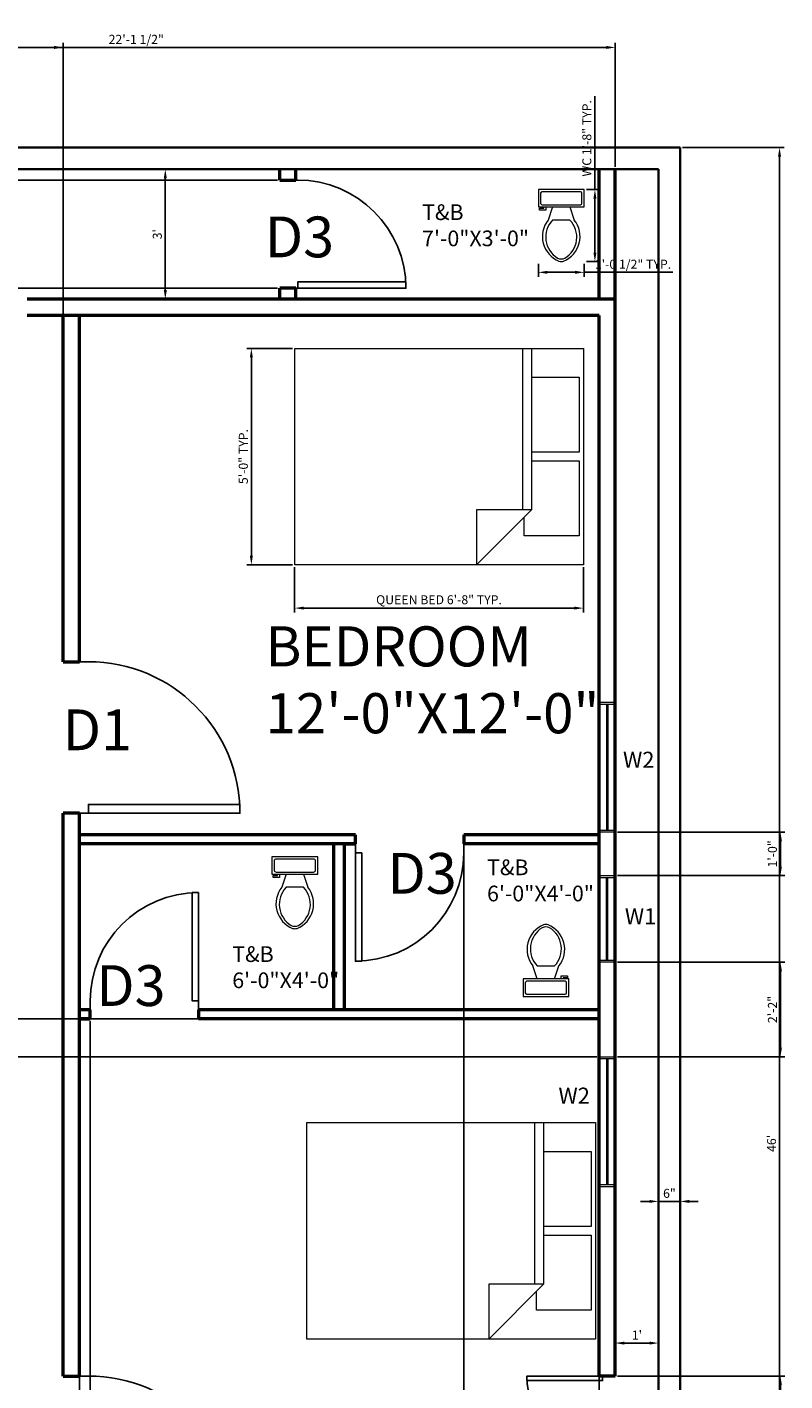
# Model space of a CAD drawing. Units: inches. Extents: x 2727 to 5054, y 1285 to 3233.
# Tile 3 of 3: x 2903 to 3113, y 1525 to 1900. Entities that reach past the tile are written whole.
import ezdxf

# ---------------------------------------------------------------- set-up
doc = ezdxf.new("R2010")
doc.units = ezdxf.units.IN
for name, color, linetype, lineweight in [('A-ANNO-TEXT', 1, 'Continuous', 18), ('A-AREA-IDEN', 1, 'Continuous', 18), ('A-FLOR-FIXT', 8, 'Continuous', 18), ('A-WALL-SITE', 7, 'Continuous', 35), ('DIMENSIONS', 9, 'Continuous', 18), ('doors', 5, 'Continuous', 25), ('furniture', 8, 'Continuous', 18), ('walls', 7, 'Continuous', 50), ('windows', 3, 'Continuous', 18)]:
    doc.layers.add(name, color=color, linetype=linetype, lineweight=lineweight)
doc.styles.get("Standard").update_dxf_attribs({"font": 'arial.ttf'})
doc.dimstyles.new('ISO-25', dxfattribs={"dimtxt": 2.5, "dimasz": 2.5, "dimexe": 1.25, "dimexo": 0.625, "dimtad": 1, "dimlunit": 4, "dimtxsty": 'Standard', "dimcen": 2.5, "dimadec": 0, "dimazin": 0, "dimtfac": 1, "dimtmove": 0, "dimatfit": 3, "dimfxl": 1, "dimarcsym": 0})

# ---------------------------------------------------------------- blocks, each defined once
blk = doc.blocks.new('*U2')
for p, q in [((0, 0), (0, -5)), ((30, 0), (30, -5))]:
    blk.add_line(p, q)
blk.add_lwpolyline([(0, 0), (0, 30), (1.75, 30), (1.75, 0)], close=True)
blk.add_arc((0, 0), 30, 0, 90)
blk = doc.blocks.new('Bed - Queen')
for p, q in [((0, -80.00003), (0, 0)), ((0, 0), (59.99999, 0)), ((59.99999, 0), (59.99999, -80.00003)), ((7.99999, -1.2), (28.79998, -1.2)), ((7.99999, -14.4), (7.99999, -1.2)), ((28.79998, -1.2), (28.79998, -14.4)), ((31.19999, -1.2), (51.99999, -1.2)), ((31.19999, -14.4), (31.19999, -1.2)), ((51.99999, -1.2), (51.99999, -16.4)), ((0, -14.4), (44.8, -14.4)), ((59.99999, -29.6), (44.8, -14.4)), ((44.8, -14.4), (44.8, -29.6)), ((44.8, -16.8), (0, -16.8)), ((51.99999, -16.4), (46.79936, -16.4)), ((44.8, -29.6), (59.99999, -29.6)), ((59.99999, -80.00003), (0, -80.00003))]:
    blk.add_line(p, q)
blk = doc.blocks.new('Toilet - top')
for p, q in [((9.5, -6), (9.5, -2)), ((-10, -8.5), (-8, -8.5)), ((-10, -9.5), (-10, -8.5)), ((-7, -9.5), (-10, -9.5)), ((-8, -8.5), (-8, -8)), ((-7, -8), (-7, -9.5)), ((-4, -8), (-6, -14)), ((4, -8), (6, -14)), ((4, -14), (-4, -14))]:
    blk.add_line(p, q)
blk.add_lwpolyline([(10.5, -8), (10.5, 0), (-10.5, 0), (-10.5, -8)], close=True)
for points in [[(-9.5, -2), (-9.5, -6)], [(8.5, -1), (-8.5, -1)], [(-8.5, -7), (8.5, -7)]]:
    blk.add_lwpolyline(points)
for centre, radius, start, end in [((-8.62, -1.88), 0.884, 81.8699, 188.1301), ((-8.62, -6.12), 0.884, 171.8699, 278.1301), ((8.62, -1.88), 0.884, 351.8699, 98.1301), ((8.62, -6.12), 0.884, 261.8699, 8.1301), ((3.52, -21.58), 12.17, 141.46911, 247.97143), ((4.2, -21.82), 11.33, 136.36773, 238.94682), ((-3.52, -21.58), 12.17, 292.02843, 38.53071), ((-4.2, -21.82), 11.33, 301.05301, 43.63209), ((0, -27.88), 4, 245.73182, 294.26817), ((0, -29), 4, 254.86053, 285.13947)]:
    blk.add_arc(centre, radius, start, end)
blk = doc.blocks.new('*D9')
at = {"layer": 'Defpoints', "color": 0, "transparency": 16777216}
for p in [(3084.39, 1866.39), (3084.39, 1314.39), (3111.91, 1314.39)]:
    blk.add_point(p, dxfattribs=at)
at = {"layer": 'DIMENSIONS', "color": 0, "lineweight": -2, "transparency": 16777216}
for p, q in [((3085.02, 1866.39), (3113.16, 1866.39)), ((3111.91, 1863.89), (3111.91, 1316.89)), ((3085.02, 1314.39), (3113.16, 1314.39))]:
    blk.add_line(p, q, dxfattribs=at)
at = {"layer": 'DIMENSIONS', "color": 0, "transparency": 16777216}
for points in [[(3111.49, 1863.89), (3112.33, 1863.89), (3111.91, 1866.39)], [(3111.49, 1316.89), (3112.33, 1316.89), (3111.91, 1314.39)]]:
    blk.add_solid(points, dxfattribs=at)
at = {"layer": 'DIMENSIONS', "color": 0, "transparency": 16777216, "insert": (3110.01, 1590.39), "char_height": 2.5, "attachment_point": 5, "rotation": 90}
blk.add_mtext("46'", dxfattribs=at)
blk = doc.blocks.new('*D11')
at = {"layer": 'Defpoints', "color": 0, "transparency": 16777216}
for p in [(3078.39, 1577.87), (3084.39, 1577.87), (3084.39, 1574.3)]:
    blk.add_point(p, dxfattribs=at)
at = {"layer": 'DIMENSIONS', "color": 0, "lineweight": -2, "transparency": 16777216}
for p, q in [((3078.39, 1577.25), (3078.39, 1573.05)), ((3084.39, 1577.25), (3084.39, 1573.05)), ((3075.89, 1574.3), (3073.39, 1574.3)), ((3078.39, 1574.3), (3084.39, 1574.3)), ((3086.89, 1574.3), (3089.39, 1574.3))]:
    blk.add_line(p, q, dxfattribs=at)
at = {"layer": 'DIMENSIONS', "color": 0, "transparency": 16777216}
for points in [[(3075.89, 1574.72), (3075.89, 1573.89), (3078.39, 1574.3)], [(3086.89, 1574.72), (3086.89, 1573.89), (3084.39, 1574.3)]]:
    blk.add_solid(points, dxfattribs=at)
at = {"layer": 'DIMENSIONS', "color": 0, "transparency": 16777216, "insert": (3081.39, 1576.21), "char_height": 2.5, "attachment_point": 5}
blk.add_mtext('6"', dxfattribs=at)
blk = doc.blocks.new('*D12')
at = {"layer": 'Defpoints', "color": 0, "transparency": 16777216}
for p in [(3066.39, 1535.04), (3078.39, 1535.04), (3078.39, 1535.04)]:
    blk.add_point(p, dxfattribs=at)
at = {"layer": 'DIMENSIONS', "color": 0, "lineweight": -2, "transparency": 16777216}
for p, q in [((3066.39, 1535.66), (3066.39, 1536.29)), ((3068.89, 1535.04), (3075.89, 1535.04)), ((3078.39, 1535.66), (3078.39, 1536.29))]:
    blk.add_line(p, q, dxfattribs=at)
at = {"layer": 'DIMENSIONS', "color": 0, "transparency": 16777216}
for points in [[(3068.89, 1535.45), (3068.89, 1534.62), (3066.39, 1535.04)], [(3075.89, 1535.45), (3075.89, 1534.62), (3078.39, 1535.04)]]:
    blk.add_solid(points, dxfattribs=at)
at = {"layer": 'DIMENSIONS', "color": 0, "transparency": 16777216, "insert": (3072.39, 1536.92), "char_height": 2.5, "attachment_point": 5}
blk.add_mtext("1'", dxfattribs=at)
blk = doc.blocks.new('*D13')
at = {"layer": 'Defpoints', "color": 0, "transparency": 16777216}
for p in [(2935.22, 1860.39), (2935.22, 1824.39), (2941.69, 1824.39)]:
    blk.add_point(p, dxfattribs=at)
at = {"layer": 'DIMENSIONS', "color": 0, "lineweight": -2, "transparency": 16777216}
for p, q in [((2935.84, 1860.39), (2942.94, 1860.39)), ((2941.69, 1857.89), (2941.69, 1826.89)), ((2935.84, 1824.39), (2942.94, 1824.39))]:
    blk.add_line(p, q, dxfattribs=at)
at = {"layer": 'DIMENSIONS', "color": 0, "transparency": 16777216}
for points in [[(2941.28, 1857.89), (2942.11, 1857.89), (2941.69, 1860.39)], [(2941.28, 1826.89), (2942.11, 1826.89), (2941.69, 1824.39)]]:
    blk.add_solid(points, dxfattribs=at)
at = {"layer": 'DIMENSIONS', "color": 0, "transparency": 16777216, "insert": (2939.79, 1842.39), "char_height": 2.5, "attachment_point": 5, "rotation": 90}
blk.add_mtext("3'", dxfattribs=at)
blk = doc.blocks.new('WIN-W1-24IN')
for p, q in [((0, 4.5), (24.02, 4.5)), ((0, 0), (0, 4.5)), ((0.5, 0), (0.5, 4.5)), ((23.52, 4.5), (23.52, 0)), ((24.02, 4.5), (24.02, 0)), ((24.02, 0), (0, 0)), ((0.5, 2.45), (23.52, 2.45)), ((0.5, 2.05), (23.52, 2.05))]:
    blk.add_line(p, q)
blk = doc.blocks.new('WIN-W2-36IN')
for p, q in [((0, 0), (0, 36.02)), ((0, 36.02), (4.5, 36.02)), ((0, 35.52), (4.5, 35.52)), ((2.05, 35.52), (2.05, 0.5)), ((2.45, 35.52), (2.45, 0.5)), ((4.5, 36.02), (4.5, 0)), ((4.5, 0.5), (0, 0.5)), ((4.5, 0), (0, 0))]:
    blk.add_line(p, q)
blk = doc.blocks.new('*D31')
at = {"layer": 'Defpoints', "color": 0, "transparency": 16777216}
for p in [(3057.76, 1854.77), (3060.75, 1854.77), (3057.76, 1834.81)]:
    blk.add_point(p, dxfattribs=at)
at = {"layer": 'DIMENSIONS', "color": 0, "lineweight": -2, "transparency": 16777216}
for p, q in [((3060.75, 1854.77), (3060.75, 1880.65)), ((3058.38, 1854.77), (3062, 1854.77)), ((3060.75, 1837.31), (3060.75, 1852.27)), ((3058.38, 1834.81), (3062, 1834.81))]:
    blk.add_line(p, q, dxfattribs=at)
at = {"layer": 'DIMENSIONS', "color": 0, "transparency": 16777216}
for points in [[(3060.33, 1852.27), (3061.17, 1852.27), (3060.75, 1854.77)], [(3060.33, 1837.31), (3061.17, 1837.31), (3060.75, 1834.81)]]:
    blk.add_solid(points, dxfattribs=at)
at = {"layer": 'DIMENSIONS', "color": 0, "transparency": 16777216, "insert": (3058.83, 1868.96), "char_height": 2.5, "attachment_point": 5, "rotation": 90}
blk.add_mtext('WC 1\'-8" TYP.', dxfattribs=at)
blk = doc.blocks.new('*D32')
at = {"layer": 'Defpoints', "color": 0, "transparency": 16777216}
for p in [(3045.08, 1834.81), (3057.76, 1834.81), (3057.76, 1831.82)]:
    blk.add_point(p, dxfattribs=at)
at = {"layer": 'DIMENSIONS', "color": 0, "lineweight": -2, "transparency": 16777216}
for p, q in [((3045.08, 1834.19), (3045.08, 1830.57)), ((3047.58, 1831.82), (3055.26, 1831.82)), ((3057.76, 1834.19), (3057.76, 1830.57)), ((3057.76, 1831.82), (3082.34, 1831.82))]:
    blk.add_line(p, q, dxfattribs=at)
at = {"layer": 'DIMENSIONS', "color": 0, "transparency": 16777216}
for points in [[(3047.58, 1832.24), (3047.58, 1831.4), (3045.08, 1831.82)], [(3055.26, 1832.24), (3055.26, 1831.4), (3057.76, 1831.82)]]:
    blk.add_solid(points, dxfattribs=at)
at = {"layer": 'DIMENSIONS', "color": 0, "transparency": 16777216, "insert": (3071.3, 1833.74), "char_height": 2.5, "attachment_point": 5}
blk.add_mtext('1\'-0 1/2" TYP.', dxfattribs=at)
blk = doc.blocks.new('*D33')
at = {"layer": 'Defpoints', "color": 0, "transparency": 16777216}
for p in [(2977.54, 1750.75), (3057.54, 1750.75), (3057.54, 1738.75)]:
    blk.add_point(p, dxfattribs=at)
at = {"layer": 'DIMENSIONS', "color": 0, "lineweight": -2, "transparency": 16777216}
for p, q in [((2977.54, 1750.12), (2977.54, 1737.5)), ((3057.54, 1750.12), (3057.54, 1737.5)), ((2980.04, 1738.75), (3055.04, 1738.75))]:
    blk.add_line(p, q, dxfattribs=at)
at = {"layer": 'DIMENSIONS', "color": 0, "transparency": 16777216}
for points in [[(2980.04, 1739.16), (2980.04, 1738.33), (2977.54, 1738.75)], [(3055.04, 1739.16), (3055.04, 1738.33), (3057.54, 1738.75)]]:
    blk.add_solid(points, dxfattribs=at)
at = {"layer": 'DIMENSIONS', "color": 0, "transparency": 16777216, "insert": (3017.54, 1740.74), "char_height": 2.5, "attachment_point": 5}
blk.add_mtext('QUEEN BED 6\'-8" TYP.', dxfattribs=at)
blk = doc.blocks.new('*D34')
at = {"layer": 'Defpoints', "color": 0, "transparency": 16777216}
for p in [(2977.54, 1810.75), (2965.54, 1750.75), (2977.54, 1750.75)]:
    blk.add_point(p, dxfattribs=at)
at = {"layer": 'DIMENSIONS', "color": 0, "lineweight": -2, "transparency": 16777216}
for p, q in [((2976.92, 1810.75), (2964.29, 1810.75)), ((2965.54, 1808.25), (2965.54, 1753.25)), ((2976.92, 1750.75), (2964.29, 1750.75))]:
    blk.add_line(p, q, dxfattribs=at)
at = {"layer": 'DIMENSIONS', "color": 0, "transparency": 16777216}
for points in [[(2965.13, 1808.25), (2965.96, 1808.25), (2965.54, 1810.75)], [(2965.13, 1753.25), (2965.96, 1753.25), (2965.54, 1750.75)]]:
    blk.add_solid(points, dxfattribs=at)
at = {"layer": 'DIMENSIONS', "color": 0, "transparency": 16777216, "insert": (2963.64, 1780.75), "char_height": 2.5, "attachment_point": 5, "rotation": 90}
blk.add_mtext('5\'-0" TYP.', dxfattribs=at)
blk = doc.blocks.new('*D41')
at = {"layer": 'Defpoints', "color": 0, "transparency": 16777216}
for p in [(3066.39, 1894.15), (3066.39, 1860.39), (2800.89, 1824.39)]:
    blk.add_point(p, dxfattribs=at)
at = {"layer": 'DIMENSIONS', "color": 0, "lineweight": -2, "transparency": 16777216}
for p, q in [((2800.89, 1825.02), (2800.89, 1895.4)), ((3066.39, 1861.02), (3066.39, 1895.4)), ((2803.39, 1894.15), (3063.89, 1894.15))]:
    blk.add_line(p, q, dxfattribs=at)
at = {"layer": 'DIMENSIONS', "color": 0, "transparency": 16777216}
for points in [[(2803.39, 1894.57), (2803.39, 1893.73), (2800.89, 1894.15)], [(3063.89, 1894.57), (3063.89, 1893.73), (3066.39, 1894.15)]]:
    blk.add_solid(points, dxfattribs=at)
at = {"layer": 'DIMENSIONS', "color": 0, "transparency": 16777216, "insert": (2933.64, 1896.07), "char_height": 2.5, "attachment_point": 5}
blk.add_mtext('22\'-1 1/2"', dxfattribs=at)
blk = doc.blocks.new('*D45')
at = {"layer": 'Defpoints', "color": 0, "transparency": 16777216}
for p in [(2732.63, 1857.39), (2973.39, 1857.39), (2973.39, 1827.39)]:
    blk.add_point(p, dxfattribs=at)
at = {"layer": 'DIMENSIONS', "color": 0, "lineweight": -2, "transparency": 16777216}
for p, q in [((2972.77, 1857.39), (2731.38, 1857.39)), ((2732.63, 1829.89), (2732.63, 1854.89)), ((2972.77, 1827.39), (2731.38, 1827.39))]:
    blk.add_line(p, q, dxfattribs=at)
at = {"layer": 'DIMENSIONS', "color": 0, "transparency": 16777216}
for points in [[(2732.21, 1854.89), (2733.05, 1854.89), (2732.63, 1857.39)], [(2732.21, 1829.89), (2733.05, 1829.89), (2732.63, 1827.39)]]:
    blk.add_solid(points, dxfattribs=at)
at = {"layer": 'DIMENSIONS', "color": 0, "transparency": 16777216, "insert": (2730.73, 1842.39), "char_height": 2.5, "attachment_point": 5, "rotation": 90}
blk.add_mtext('2\'-6"', dxfattribs=at)
blk = doc.blocks.new('*D56')
at = {"layer": 'Defpoints', "color": 0, "transparency": 16777216}
for p in [(2913.39, 1894.15), (2877.39, 1728.39), (2913.39, 1723.89)]:
    blk.add_point(p, dxfattribs=at)
at = {"layer": 'DIMENSIONS', "color": 0, "lineweight": -2, "transparency": 16777216}
for p, q in [((2877.39, 1729.02), (2877.39, 1895.4)), ((2913.39, 1724.52), (2913.39, 1895.4)), ((2879.89, 1894.15), (2910.89, 1894.15))]:
    blk.add_line(p, q, dxfattribs=at)
at = {"layer": 'DIMENSIONS', "color": 0, "transparency": 16777216}
for points in [[(2879.89, 1894.57), (2879.89, 1893.73), (2877.39, 1894.15)], [(2910.89, 1894.57), (2910.89, 1893.73), (2913.39, 1894.15)]]:
    blk.add_solid(points, dxfattribs=at)
at = {"layer": 'DIMENSIONS', "color": 0, "transparency": 16777216, "insert": (2895.39, 1896.05), "char_height": 2.5, "attachment_point": 5}
blk.add_mtext('3\'-0"', dxfattribs=at)
blk = doc.blocks.new('*D57')
at = {"layer": 'Defpoints', "color": 0, "transparency": 16777216}
for p in [(3066.39, 1525.89), (3112.15, 1525.89), (3066.39, 1483.89)]:
    blk.add_point(p, dxfattribs=at)
at = {"layer": 'DIMENSIONS', "color": 0, "lineweight": -2, "transparency": 16777216}
for p, q in [((3067.02, 1525.89), (3113.4, 1525.89)), ((3112.15, 1486.39), (3112.15, 1523.39)), ((3067.02, 1483.89), (3113.4, 1483.89))]:
    blk.add_line(p, q, dxfattribs=at)
at = {"layer": 'DIMENSIONS', "color": 0, "transparency": 16777216}
for points in [[(3111.73, 1523.39), (3112.57, 1523.39), (3112.15, 1525.89)], [(3111.73, 1486.39), (3112.57, 1486.39), (3112.15, 1483.89)]]:
    blk.add_solid(points, dxfattribs=at)
at = {"layer": 'DIMENSIONS', "color": 0, "transparency": 16777216, "insert": (3110.25, 1504.89), "char_height": 2.5, "attachment_point": 5, "rotation": 90}
blk.add_mtext('3\'-6"', dxfattribs=at)
blk = doc.blocks.new('*D58')
at = {"layer": 'Defpoints', "color": 0, "transparency": 16777216}
for p in [(2732.63, 1624.89), (3061.89, 1624.89), (3061.89, 1614.39)]:
    blk.add_point(p, dxfattribs=at)
at = {"layer": 'DIMENSIONS', "color": 0, "lineweight": -2, "transparency": 16777216}
for p, q in [((2732.63, 1624.89), (2732.63, 1643.05)), ((3061.27, 1624.89), (2731.38, 1624.89)), ((2732.63, 1616.89), (2732.63, 1622.39)), ((3061.27, 1614.39), (2731.38, 1614.39))]:
    blk.add_line(p, q, dxfattribs=at)
at = {"layer": 'DIMENSIONS', "color": 0, "transparency": 16777216}
for points in [[(2732.21, 1622.39), (2733.05, 1622.39), (2732.63, 1624.89)], [(2732.21, 1616.89), (2733.05, 1616.89), (2732.63, 1614.39)]]:
    blk.add_solid(points, dxfattribs=at)
at = {"layer": 'DIMENSIONS', "color": 0, "transparency": 16777216, "insert": (2730.71, 1635.22), "char_height": 2.5, "attachment_point": 5, "rotation": 90}
blk.add_mtext('0\'-10 1/2"', dxfattribs=at)
blk = doc.blocks.new('*D59')
at = {"layer": 'Defpoints', "color": 0, "transparency": 16777216}
for p in [(3066.39, 1640.59), (3112.15, 1640.59), (3066.39, 1614.39)]:
    blk.add_point(p, dxfattribs=at)
at = {"layer": 'DIMENSIONS', "color": 0, "lineweight": -2, "transparency": 16777216}
for p, q in [((3067.02, 1640.59), (3113.4, 1640.59)), ((3112.15, 1616.89), (3112.15, 1638.09)), ((3067.02, 1614.39), (3113.4, 1614.39))]:
    blk.add_line(p, q, dxfattribs=at)
at = {"layer": 'DIMENSIONS', "color": 0, "transparency": 16777216}
for points in [[(3111.73, 1638.09), (3112.57, 1638.09), (3112.15, 1640.59)], [(3111.73, 1616.89), (3112.57, 1616.89), (3112.15, 1614.39)]]:
    blk.add_solid(points, dxfattribs=at)
at = {"layer": 'DIMENSIONS', "color": 0, "transparency": 16777216, "insert": (3110.27, 1627.49), "char_height": 2.5, "attachment_point": 5, "rotation": 90}
blk.add_mtext('2\'-2"', dxfattribs=at)
blk = doc.blocks.new('*D60')
at = {"layer": 'Defpoints', "color": 0, "transparency": 16777216}
for p in [(3066.39, 1676.63), (3112.15, 1676.63), (3066.39, 1664.61)]:
    blk.add_point(p, dxfattribs=at)
at = {"layer": 'DIMENSIONS', "color": 0, "lineweight": -2, "transparency": 16777216}
for p, q in [((3067.02, 1676.63), (3113.4, 1676.63)), ((3112.15, 1667.11), (3112.15, 1674.13)), ((3067.02, 1664.61), (3113.4, 1664.61))]:
    blk.add_line(p, q, dxfattribs=at)
at = {"layer": 'DIMENSIONS', "color": 0, "transparency": 16777216}
for points in [[(3111.73, 1674.13), (3112.57, 1674.13), (3112.15, 1676.63)], [(3111.73, 1667.11), (3112.57, 1667.11), (3112.15, 1664.61)]]:
    blk.add_solid(points, dxfattribs=at)
at = {"layer": 'DIMENSIONS', "color": 0, "transparency": 16777216, "insert": (3110.25, 1670.62), "char_height": 2.5, "attachment_point": 5, "rotation": 90}
blk.add_mtext('1\'-0"', dxfattribs=at)
blk = doc.blocks.new('*D62')
at = {"layer": 'Defpoints', "color": 0, "transparency": 16777216}
for p in [(3024.39, 1675.89), (3061.89, 1675.89), (3061.89, 1286.63)]:
    blk.add_point(p, dxfattribs=at)
at = {"layer": 'DIMENSIONS', "color": 0, "lineweight": -2, "transparency": 16777216}
for p, q in [((3024.39, 1675.27), (3024.39, 1285.38)), ((3061.89, 1675.27), (3061.89, 1285.38)), ((3026.89, 1286.63), (3059.39, 1286.63))]:
    blk.add_line(p, q, dxfattribs=at)
at = {"layer": 'DIMENSIONS', "color": 0, "transparency": 16777216}
for points in [[(3026.89, 1287.05), (3026.89, 1286.21), (3024.39, 1286.63)], [(3059.39, 1287.05), (3059.39, 1286.21), (3061.89, 1286.63)]]:
    blk.add_solid(points, dxfattribs=at)
at = {"layer": 'DIMENSIONS', "color": 0, "transparency": 16777216, "insert": (3043.14, 1288.55), "char_height": 2.5, "attachment_point": 5}
blk.add_mtext('3\'-1 1/2"', dxfattribs=at)
blk = doc.blocks.new('*D63')
at = {"layer": 'Defpoints', "color": 0, "transparency": 16777216}
for p in [(2917.89, 1624.89), (2920.89, 1624.89), (2920.89, 1286.63)]:
    blk.add_point(p, dxfattribs=at)
at = {"layer": 'DIMENSIONS', "color": 0, "lineweight": -2, "transparency": 16777216}
for p, q in [((2917.89, 1624.27), (2917.89, 1285.38)), ((2920.89, 1624.27), (2920.89, 1285.38)), ((2915.39, 1286.63), (2912.89, 1286.63)), ((2917.89, 1286.63), (2920.89, 1286.63)), ((2923.39, 1286.63), (2933.79, 1286.63))]:
    blk.add_line(p, q, dxfattribs=at)
at = {"layer": 'DIMENSIONS', "color": 0, "transparency": 16777216}
for points in [[(2915.39, 1287.05), (2915.39, 1286.21), (2917.89, 1286.63)], [(2923.39, 1287.05), (2923.39, 1286.21), (2920.89, 1286.63)]]:
    blk.add_solid(points, dxfattribs=at)
at = {"layer": 'DIMENSIONS', "color": 0, "transparency": 16777216, "insert": (2929.84, 1288.53), "char_height": 2.5, "attachment_point": 5}
blk.add_mtext('0\'-3"', dxfattribs=at)

msp = doc.modelspace()

# ---------------------------------------------------------------- linework, layer by layer
at = {"layer": 'A-WALL-SITE'}
for p, q in [((3084.39, 1866.39), (2760.39, 1866.39)), ((3084.39, 1314.39), (3084.39, 1866.39)), ((3078.39, 1860.39), (2766.39, 1860.39)), ((3078.39, 1320.39), (3078.39, 1860.39))]:
    msp.add_line(p, q, dxfattribs=at)
at = {"layer": 'walls'}
for p, q in [((2973.39, 1857.39), (2973.39, 1860.39)), ((2977.89, 1857.39), (2977.89, 1860.39)), ((3061.89, 1824.39), (3061.89, 1860.39)), ((3066.39, 1824.39), (3066.39, 1860.39)), ((2973.39, 1857.39), (2977.89, 1857.39)), ((3066.39, 1824.39), (2903.39, 1824.39)), ((2973.39, 1824.39), (2973.39, 1827.39)), ((2977.89, 1827.39), (2973.39, 1827.39)), ((2977.89, 1824.39), (2977.89, 1827.39)), ((2977.89, 1824.39), (2977.89, 1827.39)), ((3066.39, 1525.89), (3066.39, 1824.39)), ((3061.89, 1819.89), (2903.39, 1819.89)), ((2913.39, 1819.89), (2903.39, 1819.89)), ((2913.39, 1723.89), (2913.39, 1819.89)), ((2917.89, 1723.89), (2917.89, 1819.89)), ((3061.89, 1525.89), (3061.89, 1819.89)), ((2913.39, 1723.89), (2917.89, 1723.89)), ((2913.39, 1525.89), (2913.39, 1681.89)), ((2917.89, 1681.89), (2913.39, 1681.89)), ((2917.89, 1525.89), (2917.89, 1681.89)), ((2994.39, 1675.89), (2917.89, 1675.89)), ((2994.39, 1673.39), (2994.39, 1675.89)), ((3061.89, 1675.89), (3024.39, 1675.89)), ((3024.39, 1675.89), (3024.39, 1673.39)), ((2994.39, 1673.39), (2917.89, 1673.39)), ((2988.39, 1627.39), (2988.39, 1673.39)), ((2991.39, 1627.39), (2991.39, 1673.39)), ((2991.39, 1673.39), (2994.39, 1673.39)), ((3061.89, 1673.39), (3024.39, 1673.39)), ((2920.89, 1627.39), (2917.89, 1627.39)), ((2917.89, 1624.89), (2920.89, 1624.89)), ((2920.89, 1624.89), (2917.89, 1624.89)), ((2920.89, 1624.89), (2920.89, 1627.39)), ((3061.89, 1627.39), (2950.89, 1627.39)), ((2950.89, 1627.39), (2950.89, 1624.89)), ((3061.89, 1624.89), (2950.89, 1624.89)), ((2913.39, 1525.89), (2917.89, 1525.89)), ((3066.39, 1525.89), (3061.89, 1525.89))]:
    msp.add_line(p, q, dxfattribs=at)

# ---------------------------------------------------------------- block references
at = {"layer": 'A-FLOR-FIXT', "xscale": 0.6037841857374967, "yscale": 0.6037841857374967, "zscale": 0.6037841857374967}
for p in [(3051.417, 1854.765), (2977.586, 1669.814)]:
    msp.add_blockref('Toilet - top', p, dxfattribs=at)
at = {"layer": 'A-FLOR-FIXT', "xscale": 0.6037841857374967, "yscale": 0.6037841857374967, "zscale": 0.6037841857374967, "rotation": 180}
msp.add_blockref('Toilet - top', (3047.158, 1631.125), dxfattribs=at)
at = {"layer": 'doors', "xscale": -1}
for p, rotation in [((2978.39, 1827.39), 270), ((2994.39, 1670.89), 180)]:
    msp.add_blockref('*U2', p, dxfattribs=dict(at, rotation=rotation))
at = {"layer": 'doors'}
for p, xscale, yscale, zscale, rotation in [((2920.39, 1681.89), -1.399999999999999, 1.399999999999999, 1.399999999999999, 270), ((2920.39, 1483.89), -1.399999999999999, 1.399999999999999, 1.399999999999999, 270), ((3062.89, 1525.89), -0.7, 0.7, 0.7, 90)]:
    msp.add_blockref('*U2', p, dxfattribs=dict(at, xscale=xscale, yscale=yscale, zscale=zscale, rotation=rotation))
at = {"layer": 'doors', "xscale": -1}
msp.add_blockref('*U2', (2950.89, 1629.89), dxfattribs=at)
at = {"layer": 'furniture', "rotation": 270}
for p in [(3057.544, 1810.746), (3060.927, 1596.148)]:
    msp.add_blockref('Bed - Queen', p, dxfattribs=at)
at = {"layer": 'windows'}
for p in [(3061.89, 1676.627), (3061.89, 1578.375)]:
    msp.add_blockref('WIN-W2-36IN', p, dxfattribs=at)
at = {"layer": 'windows', "rotation": 90.00000000000551}
msp.add_blockref('WIN-W1-24IN', (3066.391, 1640.592), dxfattribs=at)

# ---------------------------------------------------------------- texts
at = {"layer": 'A-ANNO-TEXT', "char_height": 11.3069, "attachment_point": 1}
for s, insert in [('D3', (2969.286, 1847.285)), ('D1', (2913.276, 1710.668)), ('D3', (3003.274, 1670.89)), ('D3', (2922.567, 1639.78))]:
    msp.add_mtext(s, dxfattribs=dict(at, insert=insert))
at = {"layer": 'A-ANNO-TEXT', "char_height": 4.4548, "attachment_point": 1}
for s, insert in [('W2', (3068.534, 1698.938)), ('W1', (3069.047, 1655.532)), ('W2', (3050.642, 1605.84))]:
    msp.add_mtext_dynamic_manual_height_columns(s, width=0.75599, gutter_width=22.274, heights=[0], dxfattribs=dict(at, insert=insert))
at = {"layer": 'A-AREA-IDEN', "attachment_point": 1}
for s, width, gutter_width, insert, char_height in [('T&B\\P7\'-0"X3\'-0"', 1.13872, 21.763, (3012.854, 1850.662), 4.35251), ('BEDROOM\\P12\'-0"X12\'-0"', 20.03048, 55.595, (2969.448, 1733.705), 11.11906), ('T&B\\P6\'-0"X4\'-0"', 1.13872, 21.763, (3030.847, 1669.077), 4.35251), ('T&B\\P6\'-0"X4\'-0"', 1.13872, 21.763, (2960.248, 1645.025), 4.35251)]:
    msp.add_mtext_dynamic_manual_height_columns(s, width=width, gutter_width=gutter_width, heights=[0], dxfattribs=dict(at, insert=insert, char_height=char_height))

# ---------------------------------------------------------------- dimensions: what is measured, and where the dimension line sits
at = {"layer": 'DIMENSIONS'}
for base, p1, p2, override, picture, middle in [((3066.39, 1894.15), (2800.89, 1824.39), (3066.39, 1860.39), {"dimdec": 1, "dimlfac": 1, "dimrnd": 0, "dimzin": 1, "dimdsep": 46, "dimlunit": 4, "dimfrac": 2}, '*D41', (2933.64, 1896.068)), ((2913.39, 1894.15), (2877.39, 1728.39), (2913.39, 1723.89), {"dimdec": 1, "dimlfac": 1, "dimrnd": 0, "dimzin": 1, "dimdsep": 46, "dimlunit": 4, "dimfrac": 2}, '*D56', (2895.39, 1896.052)), ((3061.89, 1286.63), (3024.39, 1675.89), (3061.89, 1675.89), {"dimdec": 1, "dimlfac": 1, "dimrnd": 0, "dimzin": 1, "dimdsep": 46, "dimlunit": 4, "dimfrac": 2}, '*D62', (3043.14, 1288.549)), ((2920.89, 1286.63), (2917.89, 1624.89), (2920.89, 1624.89), {"dimdec": 1, "dimlfac": 1, "dimrnd": 0, "dimzin": 1, "dimdsep": 46, "dimlunit": 4, "dimfrac": 2}, '*D63', (2929.838, 1288.532)), ((3084.39, 1574.304), (3078.39, 1577.874), (3084.39, 1577.874), {"dimclrd": 0, "dimclre": 0, "dimclrt": 0}, '*D11', (3081.39, 1576.206)), ((3078.39, 1535.037), (3066.39, 1535.037), (3078.39, 1535.037), {"dimclrd": 0, "dimclre": 0, "dimclrt": 0}, '*D12', (3072.39, 1536.917))]:
    dim = msp.add_linear_dim(base=base, p1=p1, p2=p2, dimstyle='ISO-25', override=override, dxfattribs=at)
    dim.commit()
    dim.dimension.update_dxf_attribs({"geometry": picture, "text_midpoint": middle})
for base, p1, p2, angle, text, picture, middle in [((3060.749, 1854.765), (3057.756, 1834.813), (3057.756, 1854.765), 90, 'WC <> TYP.', '*D31', (3058.832, 1868.955)), ((2965.544, 1750.746), (2977.544, 1810.746), (2977.544, 1750.746), 270, '<> TYP.', '*D34', (2963.643, 1780.746))]:
    dim = msp.add_linear_dim(base=base, p1=p1, p2=p2, angle=angle, text=text, dimstyle='ISO-25', override={"dimdec": 1, "dimlfac": 1, "dimrnd": 0, "dimzin": 1, "dimdsep": 46, "dimlunit": 4, "dimfrac": 2}, dxfattribs=at)
    dim.commit()
    dim.dimension.update_dxf_attribs({"geometry": picture, "text_midpoint": middle})
for base, p1, p2, override, picture, middle in [((3111.911, 1314.39), (3084.39, 1866.39), (3084.39, 1314.39), {"dimclrd": 0, "dimclre": 0, "dimclrt": 0}, '*D9', (3110.01, 1590.39)), ((2941.694, 1824.39), (2935.22, 1860.39), (2935.22, 1824.39), {"dimclrd": 0, "dimclre": 0, "dimclrt": 0}, '*D13', (2939.791, 1842.39)), ((2732.63, 1857.39), (2973.39, 1827.39), (2973.39, 1857.39), {"dimdec": 1, "dimlfac": 1, "dimrnd": 0, "dimzin": 1, "dimdsep": 46, "dimlunit": 4, "dimfrac": 2}, '*D45', (2730.729, 1842.39)), ((3112.15, 1676.627), (3066.39, 1664.607), (3066.39, 1676.627), {"dimdec": 1, "dimlfac": 1, "dimrnd": 0, "dimzin": 1, "dimdsep": 46, "dimlunit": 4, "dimfrac": 2}, '*D60', (3110.249, 1670.617)), ((2732.63, 1624.89), (3061.89, 1614.39), (3061.89, 1624.89), {"dimdec": 1, "dimlfac": 1, "dimrnd": 0, "dimzin": 1, "dimdsep": 46, "dimlunit": 4, "dimfrac": 2}, '*D58', (2730.713, 1635.222)), ((3112.15, 1640.591), (3066.39, 1614.39), (3066.39, 1640.591), {"dimdec": 1, "dimlfac": 1, "dimrnd": 0, "dimzin": 1, "dimdsep": 46, "dimlunit": 4, "dimfrac": 2}, '*D59', (3110.27, 1627.491)), ((3112.15, 1525.89), (3066.39, 1483.89), (3066.39, 1525.89), {"dimdec": 1, "dimlfac": 1, "dimrnd": 0, "dimzin": 1, "dimdsep": 46, "dimlunit": 4, "dimfrac": 2}, '*D57', (3110.248, 1504.89))]:
    dim = msp.add_linear_dim(base=base, p1=p1, p2=p2, angle=90, dimstyle='ISO-25', override=override, dxfattribs=at)
    dim.commit()
    dim.dimension.update_dxf_attribs({"geometry": picture, "text_midpoint": middle})
for base, p1, p2, text, picture, middle in [((3057.756, 1831.82), (3045.077, 1834.813), (3057.756, 1834.813), '<> TYP.', '*D32', (3071.296, 1833.737)), ((3057.544, 1738.746), (2977.544, 1750.746), (3057.544, 1750.746), 'QUEEN BED <> TYP.', '*D33', (3017.544, 1740.741))]:
    dim = msp.add_linear_dim(base=base, p1=p1, p2=p2, text=text, dimstyle='ISO-25', override={"dimdec": 1, "dimlfac": 1, "dimrnd": 0, "dimzin": 1, "dimdsep": 46, "dimlunit": 4, "dimfrac": 2}, dxfattribs=at)
    dim.commit()
    dim.dimension.update_dxf_attribs({"geometry": picture, "text_midpoint": middle})

doc.saveas('drawing.dxf')
